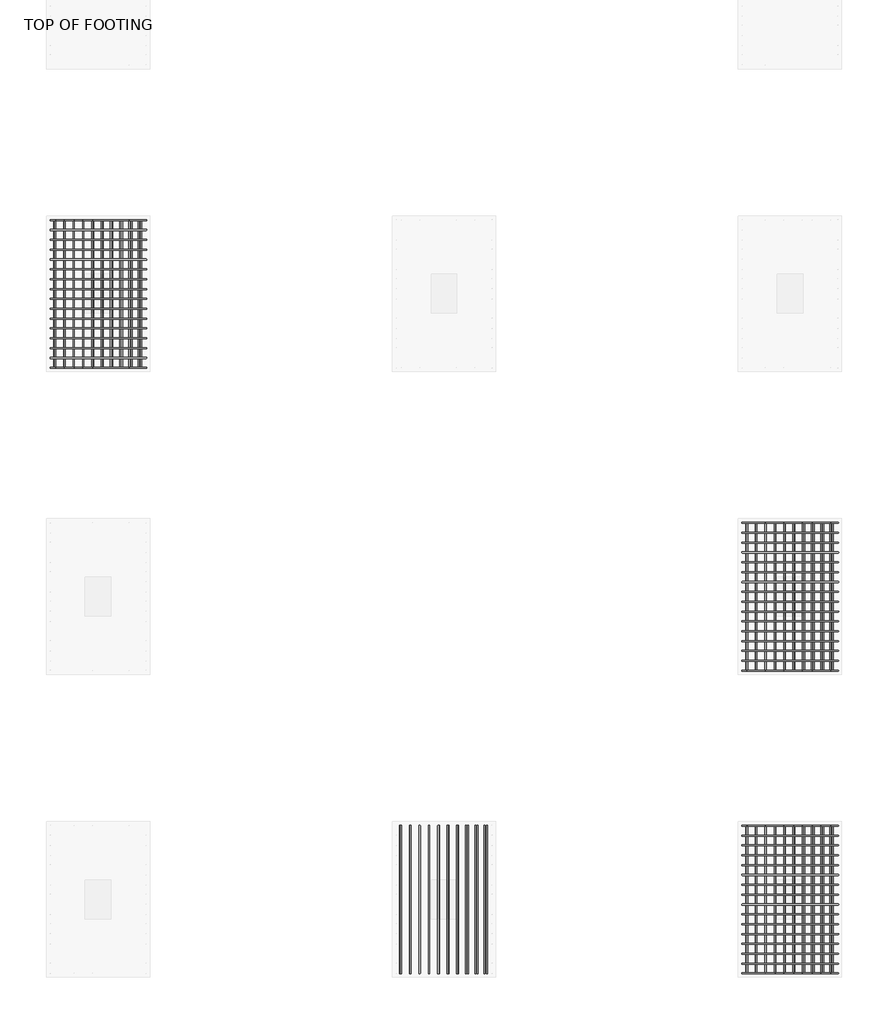
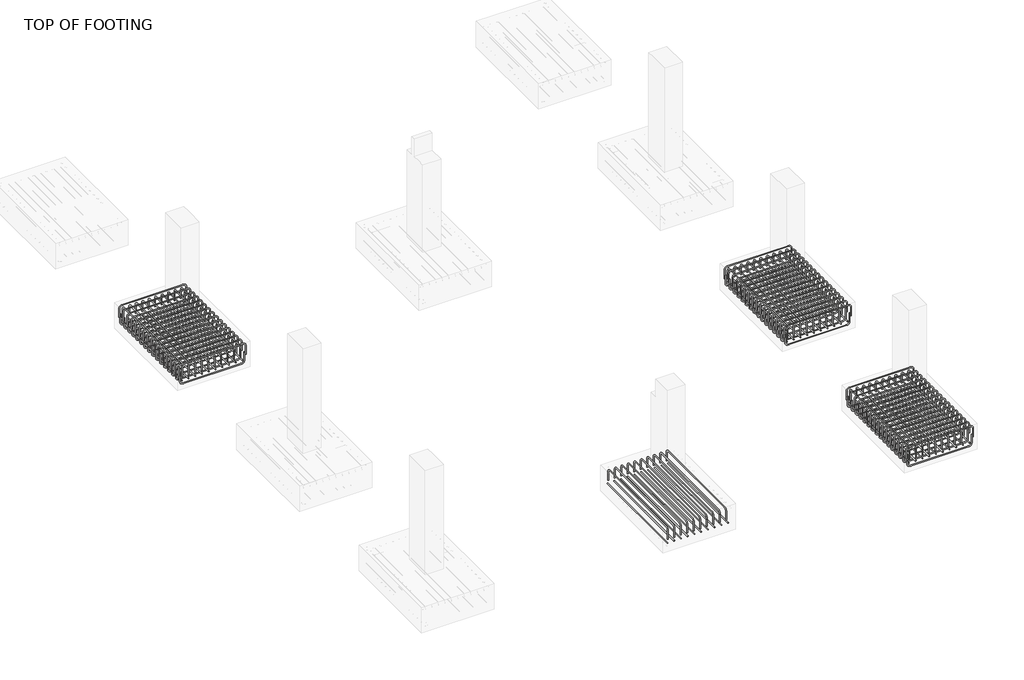
# One storey, part 6 of 8: 14 reinforcing bars.
"""IFC4 building model written with IfcOpenShell, lengths in millimetres."""

from ifc_helpers import new_model, si_unit, point, frame, origin, place, context, project, spatial, polyline, circle_curve, trimmed, segment, composite_curve, source, transform, mapped, element, save
from ifc_brep_helpers import swept_disk

model = new_model("IFC4")

# Units and contexts
model_context = context("Model", 3, world=origin())
ifc_project = project(units=[si_unit("LENGTHUNIT", "METRE", prefix="MILLI")], contexts=[model_context])

# Site, building, storey
site = spatial("IfcSite", under=ifc_project)
building = spatial("IfcBuilding", under=site)
storey = spatial("IfcBuildingStorey", under=building, Name="TOP OF FOOTING", Elevation=-1828.8)

# Reinforcing bars
placement = place(None, origin())
reinforcing_bar_shape = source(origin(), model_context, "Body", "SolidModel", [
    swept_disk(composite_curve([segment(polyline([(4698.4779803, 9626.3508557, -2021.4413313), (4698.4779803, 9626.3508557, -2168.7413313)]), True, "CONTINUOUS"), segment(trimmed(circle_curve(frame((4652.1279803, 9626.3508557, -2168.7413313), z_axis=(0.0, 1.0, 0.0), x_axis=(46.350000000000364, 0.0, 0.0)), 46.35), [point((4698.4779803, 9626.3508557, -2168.7413313))], [point((4652.1279803, 9626.3508557, -2215.0913313))], True, "CARTESIAN"), True, "CONTINUOUS"), segment(polyline([(4652.1279803, 9626.3508557, -2215.0913313), (3679.832969, 9626.3508557, -2215.0913313)]), True, "CONTINUOUS"), segment(trimmed(circle_curve(frame((3679.832969, 9626.3508557, -2168.7413313), z_axis=(0.0, 1.0, 0.0), x_axis=(0.0, 0.0, -46.34999999999991)), 46.35), [point((3679.832969, 9626.3508557, -2215.0913313))], [point((3633.482969, 9626.3508557, -2168.7413313))], True, "CARTESIAN"), True, "CONTINUOUS"), segment(polyline([(3633.482969, 9626.3508557, -2168.7413313), (3633.482969, 9626.3508557, -2021.4413313)]), True, "CONTINUOUS")], self_intersect=False), 6.35),
])
element("IfcReinforcingBar", 1, at=placement, inside=storey, context=model_context, shape_type="MappedRepresentation", body=[
    mapped(reinforcing_bar_shape, transform((0.0, 0.0, 0.0), x_axis=(1.0, 0.0, 0.0), y_axis=(0.0, 1.0, 0.0), z_axis=(0.0, 0.0, 1.0))),
    mapped(reinforcing_bar_shape, transform((0.0, -113.82, 0.0), x_axis=(1.0, 0.0, 0.0), y_axis=(0.0, 1.0, 0.0), z_axis=(0.0, 0.0, 1.0))),
    mapped(reinforcing_bar_shape, transform((0.0, -227.64, 0.0), x_axis=(1.0, 0.0, 0.0), y_axis=(0.0, 1.0, 0.0), z_axis=(0.0, 0.0, 1.0))),
    mapped(reinforcing_bar_shape, transform((0.0, -341.46, 0.0), x_axis=(1.0, 0.0, 0.0), y_axis=(0.0, 1.0, 0.0), z_axis=(0.0, 0.0, 1.0))),
    mapped(reinforcing_bar_shape, transform((0.0, -455.28, 0.0), x_axis=(1.0, 0.0, 0.0), y_axis=(0.0, 1.0, 0.0), z_axis=(0.0, 0.0, 1.0))),
    mapped(reinforcing_bar_shape, transform((0.0, -569.1, 0.0), x_axis=(1.0, 0.0, 0.0), y_axis=(0.0, 1.0, 0.0), z_axis=(0.0, 0.0, 1.0))),
    mapped(reinforcing_bar_shape, transform((0.0, -682.92, 0.0), x_axis=(1.0, 0.0, 0.0), y_axis=(0.0, 1.0, 0.0), z_axis=(0.0, 0.0, 1.0))),
    mapped(reinforcing_bar_shape, transform((0.0, -796.74, 0.0), x_axis=(1.0, 0.0, 0.0), y_axis=(0.0, 1.0, 0.0), z_axis=(0.0, 0.0, 1.0))),
    mapped(reinforcing_bar_shape, transform((0.0, -910.56, 0.0), x_axis=(1.0, 0.0, 0.0), y_axis=(0.0, 1.0, 0.0), z_axis=(0.0, 0.0, 1.0))),
    mapped(reinforcing_bar_shape, transform((0.0, -1024.38, 0.0), x_axis=(1.0, 0.0, 0.0), y_axis=(0.0, 1.0, 0.0), z_axis=(0.0, 0.0, 1.0))),
    mapped(reinforcing_bar_shape, transform((0.0, -1138.2, 0.0), x_axis=(1.0, 0.0, 0.0), y_axis=(0.0, 1.0, 0.0), z_axis=(0.0, 0.0, 1.0))),
    mapped(reinforcing_bar_shape, transform((0.0, -1252.02, 0.0), x_axis=(1.0, 0.0, 0.0), y_axis=(0.0, 1.0, 0.0), z_axis=(0.0, 0.0, 1.0))),
    mapped(reinforcing_bar_shape, transform((0.0, -1365.84, 0.0), x_axis=(1.0, 0.0, 0.0), y_axis=(0.0, 1.0, 0.0), z_axis=(0.0, 0.0, 1.0))),
    mapped(reinforcing_bar_shape, transform((0.0, -1479.66, 0.0), x_axis=(1.0, 0.0, 0.0), y_axis=(0.0, 1.0, 0.0), z_axis=(0.0, 0.0, 1.0))),
    mapped(reinforcing_bar_shape, transform((0.0, -1593.48, 0.0), x_axis=(1.0, 0.0, 0.0), y_axis=(0.0, 1.0, 0.0), z_axis=(0.0, 0.0, 1.0))),
    mapped(reinforcing_bar_shape, transform((0.0, -1707.3, 0.0), x_axis=(1.0, 0.0, 0.0), y_axis=(0.0, 1.0, 0.0), z_axis=(0.0, 0.0, 1.0))),
])
reinforcing_bar_2_shape = source(origin(), model_context, "Body", "SolidModel", [
    swept_disk(composite_curve([segment(polyline([(3615.6625983, 9626.3508557, -2068.8), (3615.6625983, 9626.3508557, -1921.5)]), True, "CONTINUOUS"), segment(trimmed(circle_curve(frame((3662.0125983, 9626.3508557, -1921.5), z_axis=(0.0, 1.0, 0.0), x_axis=(-46.34999999999991, 0.0, 0.0)), 46.35), [point((3615.6625983, 9626.3508557, -1921.5))], [point((3662.0125983, 9626.3508557, -1875.15))], True, "CARTESIAN"), True, "CONTINUOUS"), segment(polyline([(3662.0125983, 9626.3508557, -1875.15), (4676.6125983, 9626.3508557, -1875.15)]), True, "CONTINUOUS"), segment(trimmed(circle_curve(frame((4676.6125983, 9626.3508557, -1921.5), z_axis=(0.0, 1.0, 0.0), x_axis=(0.0, 0.0, 46.34999999999991)), 46.35), [point((4676.6125983, 9626.3508557, -1875.15))], [point((4722.9625983, 9626.3508557, -1921.5))], True, "CARTESIAN"), True, "CONTINUOUS"), segment(polyline([(4722.9625983, 9626.3508557, -1921.5), (4722.9625983, 9626.3508557, -2068.8)]), True, "CONTINUOUS")], self_intersect=False), 6.35),
])
element("IfcReinforcingBar", 2, at=placement, inside=storey, context=model_context, shape_type="MappedRepresentation", body=[
    mapped(reinforcing_bar_2_shape, transform((0.0, 0.0, 0.0), x_axis=(1.0, 0.0, 0.0), y_axis=(0.0, 1.0, 0.0), z_axis=(0.0, 0.0, 1.0))),
    mapped(reinforcing_bar_2_shape, transform((0.0, -113.82, 0.0), x_axis=(1.0, 0.0, 0.0), y_axis=(0.0, 1.0, 0.0), z_axis=(0.0, 0.0, 1.0))),
    mapped(reinforcing_bar_2_shape, transform((0.0, -227.64, 0.0), x_axis=(1.0, 0.0, 0.0), y_axis=(0.0, 1.0, 0.0), z_axis=(0.0, 0.0, 1.0))),
    mapped(reinforcing_bar_2_shape, transform((0.0, -341.46, 0.0), x_axis=(1.0, 0.0, 0.0), y_axis=(0.0, 1.0, 0.0), z_axis=(0.0, 0.0, 1.0))),
    mapped(reinforcing_bar_2_shape, transform((0.0, -455.28, 0.0), x_axis=(1.0, 0.0, 0.0), y_axis=(0.0, 1.0, 0.0), z_axis=(0.0, 0.0, 1.0))),
    mapped(reinforcing_bar_2_shape, transform((0.0, -569.1, 0.0), x_axis=(1.0, 0.0, 0.0), y_axis=(0.0, 1.0, 0.0), z_axis=(0.0, 0.0, 1.0))),
    mapped(reinforcing_bar_2_shape, transform((0.0, -682.92, 0.0), x_axis=(1.0, 0.0, 0.0), y_axis=(0.0, 1.0, 0.0), z_axis=(0.0, 0.0, 1.0))),
    mapped(reinforcing_bar_2_shape, transform((0.0, -796.74, 0.0), x_axis=(1.0, 0.0, 0.0), y_axis=(0.0, 1.0, 0.0), z_axis=(0.0, 0.0, 1.0))),
    mapped(reinforcing_bar_2_shape, transform((0.0, -910.56, 0.0), x_axis=(1.0, 0.0, 0.0), y_axis=(0.0, 1.0, 0.0), z_axis=(0.0, 0.0, 1.0))),
    mapped(reinforcing_bar_2_shape, transform((0.0, -1024.38, 0.0), x_axis=(1.0, 0.0, 0.0), y_axis=(0.0, 1.0, 0.0), z_axis=(0.0, 0.0, 1.0))),
    mapped(reinforcing_bar_2_shape, transform((0.0, -1138.2, 0.0), x_axis=(1.0, 0.0, 0.0), y_axis=(0.0, 1.0, 0.0), z_axis=(0.0, 0.0, 1.0))),
    mapped(reinforcing_bar_2_shape, transform((0.0, -1252.02, 0.0), x_axis=(1.0, 0.0, 0.0), y_axis=(0.0, 1.0, 0.0), z_axis=(0.0, 0.0, 1.0))),
    mapped(reinforcing_bar_2_shape, transform((0.0, -1365.84, 0.0), x_axis=(1.0, 0.0, 0.0), y_axis=(0.0, 1.0, 0.0), z_axis=(0.0, 0.0, 1.0))),
    mapped(reinforcing_bar_2_shape, transform((0.0, -1479.66, 0.0), x_axis=(1.0, 0.0, 0.0), y_axis=(0.0, 1.0, 0.0), z_axis=(0.0, 0.0, 1.0))),
    mapped(reinforcing_bar_2_shape, transform((0.0, -1593.48, 0.0), x_axis=(1.0, 0.0, 0.0), y_axis=(0.0, 1.0, 0.0), z_axis=(0.0, 0.0, 1.0))),
    mapped(reinforcing_bar_2_shape, transform((0.0, -1707.3, 0.0), x_axis=(1.0, 0.0, 0.0), y_axis=(0.0, 1.0, 0.0), z_axis=(0.0, 0.0, 1.0))),
])
reinforcing_bar_3_shape = source(origin(), model_context, "Body", "SolidModel", [
    swept_disk(composite_curve([segment(polyline([(3660.407291, 9632.7008557, -2155.1176129), (3660.407291, 7912.7008557, -2155.1176129)]), True, "CONTINUOUS")], self_intersect=False), 6.35),
])
element("IfcReinforcingBar", 3, at=placement, inside=storey, context=model_context, shape_type="MappedRepresentation", body=[
    mapped(reinforcing_bar_3_shape, transform((0.0, 0.0, 0.0), x_axis=(1.0, 0.0, 0.0), y_axis=(0.0, 1.0, 0.0), z_axis=(0.0, 0.0, 1.0))),
    mapped(reinforcing_bar_3_shape, transform((111.602188, 0.0, 0.0), x_axis=(1.0, 0.0, 0.0), y_axis=(0.0, 1.0, 0.0), z_axis=(0.0, 0.0, 1.0))),
    mapped(reinforcing_bar_3_shape, transform((223.2043759, 0.0, 0.0), x_axis=(1.0, 0.0, 0.0), y_axis=(0.0, 1.0, 0.0), z_axis=(0.0, 0.0, 1.0))),
    mapped(reinforcing_bar_3_shape, transform((334.8065639, 0.0, 0.0), x_axis=(1.0, 0.0, 0.0), y_axis=(0.0, 1.0, 0.0), z_axis=(0.0, 0.0, 1.0))),
    mapped(reinforcing_bar_3_shape, transform((446.4087519, 0.0, 0.0), x_axis=(1.0, 0.0, 0.0), y_axis=(0.0, 1.0, 0.0), z_axis=(0.0, 0.0, 1.0))),
    mapped(reinforcing_bar_3_shape, transform((558.0109398, 0.0, 0.0), x_axis=(1.0, 0.0, 0.0), y_axis=(0.0, 1.0, 0.0), z_axis=(0.0, 0.0, 1.0))),
    mapped(reinforcing_bar_3_shape, transform((669.6131278, 0.0, 0.0), x_axis=(1.0, 0.0, 0.0), y_axis=(0.0, 1.0, 0.0), z_axis=(0.0, 0.0, 1.0))),
    mapped(reinforcing_bar_3_shape, transform((781.2153158, 0.0, 0.0), x_axis=(1.0, 0.0, 0.0), y_axis=(0.0, 1.0, 0.0), z_axis=(0.0, 0.0, 1.0))),
    mapped(reinforcing_bar_3_shape, transform((892.8175037, 0.0, 0.0), x_axis=(1.0, 0.0, 0.0), y_axis=(0.0, 1.0, 0.0), z_axis=(0.0, 0.0, 1.0))),
    mapped(reinforcing_bar_3_shape, transform((1004.4196917, 0.0, 0.0), x_axis=(1.0, 0.0, 0.0), y_axis=(0.0, 1.0, 0.0), z_axis=(0.0, 0.0, 1.0))),
])
reinforcing_bar_4_shape = source(origin(), model_context, "Body", "SolidModel", [
    swept_disk(composite_curve([segment(polyline([(4635.7348019, 9626.3508557, -2094.6521303), (4635.7348019, 9626.3508557, -1947.3521303)]), True, "CONTINUOUS"), segment(trimmed(circle_curve(frame((4635.7348019, 9580.0008557, -1947.3521303), z_axis=(1.0, 0.0, 0.0), x_axis=(0.0, 46.350000000000364, 0.0)), 46.35), [point((4635.7348019, 9626.3508557, -1947.3521303))], [point((4635.7348019, 9580.0008557, -1901.0021303))], True, "CARTESIAN"), True, "CONTINUOUS"), segment(polyline([(4635.7348019, 9580.0008557, -1901.0021303), (4635.7348019, 7965.4008557, -1901.0021303)]), True, "CONTINUOUS"), segment(trimmed(circle_curve(frame((4635.7348019, 7965.4008557, -1947.3521303), z_axis=(1.0, 0.0, 0.0), x_axis=(0.0, 0.0, 46.34999999999991)), 46.35), [point((4635.7348019, 7965.4008557, -1901.0021303))], [point((4635.7348019, 7919.0508557, -1947.3521303))], True, "CARTESIAN"), True, "CONTINUOUS"), segment(polyline([(4635.7348019, 7919.0508557, -1947.3521303), (4635.7348019, 7919.0508557, -2094.6521303)]), True, "CONTINUOUS")], self_intersect=False), 6.35),
])
element("IfcReinforcingBar", 4, at=placement, inside=storey, context=model_context, shape_type="MappedRepresentation", body=[
    mapped(reinforcing_bar_4_shape, transform((0.0, 0.0, 0.0), x_axis=(1.0, 0.0, 0.0), y_axis=(0.0, 1.0, 0.0), z_axis=(0.0, 0.0, 1.0))),
    mapped(reinforcing_bar_4_shape, transform((-107.1680233, 0.0, 0.0), x_axis=(1.0, 0.0, 0.0), y_axis=(0.0, 1.0, 0.0), z_axis=(0.0, 0.0, 1.0))),
    mapped(reinforcing_bar_4_shape, transform((-214.3360466, 0.0, 0.0), x_axis=(1.0, 0.0, 0.0), y_axis=(0.0, 1.0, 0.0), z_axis=(0.0, 0.0, 1.0))),
    mapped(reinforcing_bar_4_shape, transform((-321.5040699, 0.0, 0.0), x_axis=(1.0, 0.0, 0.0), y_axis=(0.0, 1.0, 0.0), z_axis=(0.0, 0.0, 1.0))),
    mapped(reinforcing_bar_4_shape, transform((-428.6720932, 0.0, 0.0), x_axis=(1.0, 0.0, 0.0), y_axis=(0.0, 1.0, 0.0), z_axis=(0.0, 0.0, 1.0))),
    mapped(reinforcing_bar_4_shape, transform((-535.8401165, 0.0, 0.0), x_axis=(1.0, 0.0, 0.0), y_axis=(0.0, 1.0, 0.0), z_axis=(0.0, 0.0, 1.0))),
    mapped(reinforcing_bar_4_shape, transform((-643.0081398, 0.0, 0.0), x_axis=(1.0, 0.0, 0.0), y_axis=(0.0, 1.0, 0.0), z_axis=(0.0, 0.0, 1.0))),
    mapped(reinforcing_bar_4_shape, transform((-750.176163, 0.0, 0.0), x_axis=(1.0, 0.0, 0.0), y_axis=(0.0, 1.0, 0.0), z_axis=(0.0, 0.0, 1.0))),
    mapped(reinforcing_bar_4_shape, transform((-857.3441863, 0.0, 0.0), x_axis=(1.0, 0.0, 0.0), y_axis=(0.0, 1.0, 0.0), z_axis=(0.0, 0.0, 1.0))),
    mapped(reinforcing_bar_4_shape, transform((-964.5122096, 0.0, 0.0), x_axis=(1.0, 0.0, 0.0), y_axis=(0.0, 1.0, 0.0), z_axis=(0.0, 0.0, 1.0))),
])
reinforcing_bar_5_shape = source(origin(), model_context, "Body", "SolidModel", [
    swept_disk(composite_curve([segment(polyline([(7660.407291, 2632.7008557, -2155.1176129), (7660.407291, 912.7008557, -2155.1176129)]), True, "CONTINUOUS")], self_intersect=False), 6.35),
])
element("IfcReinforcingBar", 5, at=placement, inside=storey, context=model_context, shape_type="MappedRepresentation", body=[
    mapped(reinforcing_bar_5_shape, transform((0.0, 0.0, 0.0), x_axis=(1.0, 0.0, 0.0), y_axis=(0.0, 1.0, 0.0), z_axis=(0.0, 0.0, 1.0))),
    mapped(reinforcing_bar_5_shape, transform((111.602188, 0.0, 0.0), x_axis=(1.0, 0.0, 0.0), y_axis=(0.0, 1.0, 0.0), z_axis=(0.0, 0.0, 1.0))),
    mapped(reinforcing_bar_5_shape, transform((223.2043759, 0.0, 0.0), x_axis=(1.0, 0.0, 0.0), y_axis=(0.0, 1.0, 0.0), z_axis=(0.0, 0.0, 1.0))),
    mapped(reinforcing_bar_5_shape, transform((334.8065639, 0.0, 0.0), x_axis=(1.0, 0.0, 0.0), y_axis=(0.0, 1.0, 0.0), z_axis=(0.0, 0.0, 1.0))),
    mapped(reinforcing_bar_5_shape, transform((446.4087519, 0.0, 0.0), x_axis=(1.0, 0.0, 0.0), y_axis=(0.0, 1.0, 0.0), z_axis=(0.0, 0.0, 1.0))),
    mapped(reinforcing_bar_5_shape, transform((558.0109398, 0.0, 0.0), x_axis=(1.0, 0.0, 0.0), y_axis=(0.0, 1.0, 0.0), z_axis=(0.0, 0.0, 1.0))),
    mapped(reinforcing_bar_5_shape, transform((669.6131278, 0.0, 0.0), x_axis=(1.0, 0.0, 0.0), y_axis=(0.0, 1.0, 0.0), z_axis=(0.0, 0.0, 1.0))),
    mapped(reinforcing_bar_5_shape, transform((781.2153158, 0.0, 0.0), x_axis=(1.0, 0.0, 0.0), y_axis=(0.0, 1.0, 0.0), z_axis=(0.0, 0.0, 1.0))),
    mapped(reinforcing_bar_5_shape, transform((892.8175037, 0.0, 0.0), x_axis=(1.0, 0.0, 0.0), y_axis=(0.0, 1.0, 0.0), z_axis=(0.0, 0.0, 1.0))),
    mapped(reinforcing_bar_5_shape, transform((1004.4196917, 0.0, 0.0), x_axis=(1.0, 0.0, 0.0), y_axis=(0.0, 1.0, 0.0), z_axis=(0.0, 0.0, 1.0))),
])
reinforcing_bar_6_shape = source(origin(), model_context, "Body", "SolidModel", [
    swept_disk(composite_curve([segment(polyline([(8635.7348019, 2626.3508557, -2094.6521303), (8635.7348019, 2626.3508557, -1947.3521303)]), True, "CONTINUOUS"), segment(trimmed(circle_curve(frame((8635.7348019, 2580.0008557, -1947.3521303), z_axis=(1.0, 0.0, 0.0), x_axis=(0.0, 46.34999999999991, 0.0)), 46.35), [point((8635.7348019, 2626.3508557, -1947.3521303))], [point((8635.7348019, 2580.0008557, -1901.0021303))], True, "CARTESIAN"), True, "CONTINUOUS"), segment(polyline([(8635.7348019, 2580.0008557, -1901.0021303), (8635.7348019, 965.4008557, -1901.0021303)]), True, "CONTINUOUS"), segment(trimmed(circle_curve(frame((8635.7348019, 965.4008557, -1947.3521303), z_axis=(1.0, 0.0, 0.0), x_axis=(0.0, 0.0, 46.34999999999991)), 46.35), [point((8635.7348019, 965.4008557, -1901.0021303))], [point((8635.7348019, 919.0508557, -1947.3521303))], True, "CARTESIAN"), True, "CONTINUOUS"), segment(polyline([(8635.7348019, 919.0508557, -1947.3521303), (8635.7348019, 919.0508557, -2094.6521303)]), True, "CONTINUOUS")], self_intersect=False), 6.35),
])
element("IfcReinforcingBar", 6, at=placement, inside=storey, context=model_context, shape_type="MappedRepresentation", body=[
    mapped(reinforcing_bar_6_shape, transform((0.0, 0.0, 0.0), x_axis=(1.0, 0.0, 0.0), y_axis=(0.0, 1.0, 0.0), z_axis=(0.0, 0.0, 1.0))),
    mapped(reinforcing_bar_6_shape, transform((-107.1680233, 0.0, 0.0), x_axis=(1.0, 0.0, 0.0), y_axis=(0.0, 1.0, 0.0), z_axis=(0.0, 0.0, 1.0))),
    mapped(reinforcing_bar_6_shape, transform((-214.3360466, 0.0, 0.0), x_axis=(1.0, 0.0, 0.0), y_axis=(0.0, 1.0, 0.0), z_axis=(0.0, 0.0, 1.0))),
    mapped(reinforcing_bar_6_shape, transform((-321.5040699, 0.0, 0.0), x_axis=(1.0, 0.0, 0.0), y_axis=(0.0, 1.0, 0.0), z_axis=(0.0, 0.0, 1.0))),
    mapped(reinforcing_bar_6_shape, transform((-428.6720932, 0.0, 0.0), x_axis=(1.0, 0.0, 0.0), y_axis=(0.0, 1.0, 0.0), z_axis=(0.0, 0.0, 1.0))),
    mapped(reinforcing_bar_6_shape, transform((-535.8401165, 0.0, 0.0), x_axis=(1.0, 0.0, 0.0), y_axis=(0.0, 1.0, 0.0), z_axis=(0.0, 0.0, 1.0))),
    mapped(reinforcing_bar_6_shape, transform((-643.0081398, 0.0, 0.0), x_axis=(1.0, 0.0, 0.0), y_axis=(0.0, 1.0, 0.0), z_axis=(0.0, 0.0, 1.0))),
    mapped(reinforcing_bar_6_shape, transform((-750.176163, 0.0, 0.0), x_axis=(1.0, 0.0, 0.0), y_axis=(0.0, 1.0, 0.0), z_axis=(0.0, 0.0, 1.0))),
    mapped(reinforcing_bar_6_shape, transform((-857.3441863, 0.0, 0.0), x_axis=(1.0, 0.0, 0.0), y_axis=(0.0, 1.0, 0.0), z_axis=(0.0, 0.0, 1.0))),
    mapped(reinforcing_bar_6_shape, transform((-964.5122096, 0.0, 0.0), x_axis=(1.0, 0.0, 0.0), y_axis=(0.0, 1.0, 0.0), z_axis=(0.0, 0.0, 1.0))),
])
reinforcing_bar_7_shape = source(origin(), model_context, "Body", "SolidModel", [
    swept_disk(composite_curve([segment(polyline([(12698.4779803, 6126.3508557, -2021.4413313), (12698.4779803, 6126.3508557, -2168.7413313)]), True, "CONTINUOUS"), segment(trimmed(circle_curve(frame((12652.1279803, 6126.3508557, -2168.7413313), z_axis=(0.0, 1.0, 0.0), x_axis=(46.350000000000364, 0.0, 0.0)), 46.35), [point((12698.4779803, 6126.3508557, -2168.7413313))], [point((12652.1279803, 6126.3508557, -2215.0913313))], True, "CARTESIAN"), True, "CONTINUOUS"), segment(polyline([(12652.1279803, 6126.3508557, -2215.0913313), (11679.832969, 6126.3508557, -2215.0913313)]), True, "CONTINUOUS"), segment(trimmed(circle_curve(frame((11679.832969, 6126.3508557, -2168.7413313), z_axis=(0.0, 1.0, 0.0), x_axis=(0.0, 0.0, -46.34999999999991)), 46.35), [point((11679.832969, 6126.3508557, -2215.0913313))], [point((11633.482969, 6126.3508557, -2168.7413313))], True, "CARTESIAN"), True, "CONTINUOUS"), segment(polyline([(11633.482969, 6126.3508557, -2168.7413313), (11633.482969, 6126.3508557, -2021.4413313)]), True, "CONTINUOUS")], self_intersect=False), 6.35),
])
element("IfcReinforcingBar", 7, at=placement, inside=storey, context=model_context, shape_type="MappedRepresentation", body=[
    mapped(reinforcing_bar_7_shape, transform((0.0, 0.0, 0.0), x_axis=(1.0, 0.0, 0.0), y_axis=(0.0, 1.0, 0.0), z_axis=(0.0, 0.0, 1.0))),
    mapped(reinforcing_bar_7_shape, transform((0.0, -113.82, 0.0), x_axis=(1.0, 0.0, 0.0), y_axis=(0.0, 1.0, 0.0), z_axis=(0.0, 0.0, 1.0))),
    mapped(reinforcing_bar_7_shape, transform((0.0, -227.64, 0.0), x_axis=(1.0, 0.0, 0.0), y_axis=(0.0, 1.0, 0.0), z_axis=(0.0, 0.0, 1.0))),
    mapped(reinforcing_bar_7_shape, transform((0.0, -341.46, 0.0), x_axis=(1.0, 0.0, 0.0), y_axis=(0.0, 1.0, 0.0), z_axis=(0.0, 0.0, 1.0))),
    mapped(reinforcing_bar_7_shape, transform((0.0, -455.28, 0.0), x_axis=(1.0, 0.0, 0.0), y_axis=(0.0, 1.0, 0.0), z_axis=(0.0, 0.0, 1.0))),
    mapped(reinforcing_bar_7_shape, transform((0.0, -569.1, 0.0), x_axis=(1.0, 0.0, 0.0), y_axis=(0.0, 1.0, 0.0), z_axis=(0.0, 0.0, 1.0))),
    mapped(reinforcing_bar_7_shape, transform((0.0, -682.92, 0.0), x_axis=(1.0, 0.0, 0.0), y_axis=(0.0, 1.0, 0.0), z_axis=(0.0, 0.0, 1.0))),
    mapped(reinforcing_bar_7_shape, transform((0.0, -796.74, 0.0), x_axis=(1.0, 0.0, 0.0), y_axis=(0.0, 1.0, 0.0), z_axis=(0.0, 0.0, 1.0))),
    mapped(reinforcing_bar_7_shape, transform((0.0, -910.56, 0.0), x_axis=(1.0, 0.0, 0.0), y_axis=(0.0, 1.0, 0.0), z_axis=(0.0, 0.0, 1.0))),
    mapped(reinforcing_bar_7_shape, transform((0.0, -1024.38, 0.0), x_axis=(1.0, 0.0, 0.0), y_axis=(0.0, 1.0, 0.0), z_axis=(0.0, 0.0, 1.0))),
    mapped(reinforcing_bar_7_shape, transform((0.0, -1138.2, 0.0), x_axis=(1.0, 0.0, 0.0), y_axis=(0.0, 1.0, 0.0), z_axis=(0.0, 0.0, 1.0))),
    mapped(reinforcing_bar_7_shape, transform((0.0, -1252.02, 0.0), x_axis=(1.0, 0.0, 0.0), y_axis=(0.0, 1.0, 0.0), z_axis=(0.0, 0.0, 1.0))),
    mapped(reinforcing_bar_7_shape, transform((0.0, -1365.84, 0.0), x_axis=(1.0, 0.0, 0.0), y_axis=(0.0, 1.0, 0.0), z_axis=(0.0, 0.0, 1.0))),
    mapped(reinforcing_bar_7_shape, transform((0.0, -1479.66, 0.0), x_axis=(1.0, 0.0, 0.0), y_axis=(0.0, 1.0, 0.0), z_axis=(0.0, 0.0, 1.0))),
    mapped(reinforcing_bar_7_shape, transform((0.0, -1593.48, 0.0), x_axis=(1.0, 0.0, 0.0), y_axis=(0.0, 1.0, 0.0), z_axis=(0.0, 0.0, 1.0))),
    mapped(reinforcing_bar_7_shape, transform((0.0, -1707.3, 0.0), x_axis=(1.0, 0.0, 0.0), y_axis=(0.0, 1.0, 0.0), z_axis=(0.0, 0.0, 1.0))),
])
reinforcing_bar_8_shape = source(origin(), model_context, "Body", "SolidModel", [
    swept_disk(composite_curve([segment(polyline([(11615.6625983, 6126.3508557, -2068.8), (11615.6625983, 6126.3508557, -1921.5)]), True, "CONTINUOUS"), segment(trimmed(circle_curve(frame((11662.0125983, 6126.3508557, -1921.5), z_axis=(0.0, 1.0, 0.0), x_axis=(-46.350000000000364, 0.0, 0.0)), 46.35), [point((11615.6625983, 6126.3508557, -1921.5))], [point((11662.0125983, 6126.3508557, -1875.15))], True, "CARTESIAN"), True, "CONTINUOUS"), segment(polyline([(11662.0125983, 6126.3508557, -1875.15), (12676.6125983, 6126.3508557, -1875.15)]), True, "CONTINUOUS"), segment(trimmed(circle_curve(frame((12676.6125983, 6126.3508557, -1921.5), z_axis=(0.0, 1.0, 0.0), x_axis=(0.0, 0.0, 46.34999999999991)), 46.35), [point((12676.6125983, 6126.3508557, -1875.15))], [point((12722.9625983, 6126.3508557, -1921.5))], True, "CARTESIAN"), True, "CONTINUOUS"), segment(polyline([(12722.9625983, 6126.3508557, -1921.5), (12722.9625983, 6126.3508557, -2068.8)]), True, "CONTINUOUS")], self_intersect=False), 6.35),
])
element("IfcReinforcingBar", 8, at=placement, inside=storey, context=model_context, shape_type="MappedRepresentation", body=[
    mapped(reinforcing_bar_8_shape, transform((0.0, 0.0, 0.0), x_axis=(1.0, 0.0, 0.0), y_axis=(0.0, 1.0, 0.0), z_axis=(0.0, 0.0, 1.0))),
    mapped(reinforcing_bar_8_shape, transform((0.0, -113.82, 0.0), x_axis=(1.0, 0.0, 0.0), y_axis=(0.0, 1.0, 0.0), z_axis=(0.0, 0.0, 1.0))),
    mapped(reinforcing_bar_8_shape, transform((0.0, -227.64, 0.0), x_axis=(1.0, 0.0, 0.0), y_axis=(0.0, 1.0, 0.0), z_axis=(0.0, 0.0, 1.0))),
    mapped(reinforcing_bar_8_shape, transform((0.0, -341.46, 0.0), x_axis=(1.0, 0.0, 0.0), y_axis=(0.0, 1.0, 0.0), z_axis=(0.0, 0.0, 1.0))),
    mapped(reinforcing_bar_8_shape, transform((0.0, -455.28, 0.0), x_axis=(1.0, 0.0, 0.0), y_axis=(0.0, 1.0, 0.0), z_axis=(0.0, 0.0, 1.0))),
    mapped(reinforcing_bar_8_shape, transform((0.0, -569.1, 0.0), x_axis=(1.0, 0.0, 0.0), y_axis=(0.0, 1.0, 0.0), z_axis=(0.0, 0.0, 1.0))),
    mapped(reinforcing_bar_8_shape, transform((0.0, -682.92, 0.0), x_axis=(1.0, 0.0, 0.0), y_axis=(0.0, 1.0, 0.0), z_axis=(0.0, 0.0, 1.0))),
    mapped(reinforcing_bar_8_shape, transform((0.0, -796.74, 0.0), x_axis=(1.0, 0.0, 0.0), y_axis=(0.0, 1.0, 0.0), z_axis=(0.0, 0.0, 1.0))),
    mapped(reinforcing_bar_8_shape, transform((0.0, -910.56, 0.0), x_axis=(1.0, 0.0, 0.0), y_axis=(0.0, 1.0, 0.0), z_axis=(0.0, 0.0, 1.0))),
    mapped(reinforcing_bar_8_shape, transform((0.0, -1024.38, 0.0), x_axis=(1.0, 0.0, 0.0), y_axis=(0.0, 1.0, 0.0), z_axis=(0.0, 0.0, 1.0))),
    mapped(reinforcing_bar_8_shape, transform((0.0, -1138.2, 0.0), x_axis=(1.0, 0.0, 0.0), y_axis=(0.0, 1.0, 0.0), z_axis=(0.0, 0.0, 1.0))),
    mapped(reinforcing_bar_8_shape, transform((0.0, -1252.02, 0.0), x_axis=(1.0, 0.0, 0.0), y_axis=(0.0, 1.0, 0.0), z_axis=(0.0, 0.0, 1.0))),
    mapped(reinforcing_bar_8_shape, transform((0.0, -1365.84, 0.0), x_axis=(1.0, 0.0, 0.0), y_axis=(0.0, 1.0, 0.0), z_axis=(0.0, 0.0, 1.0))),
    mapped(reinforcing_bar_8_shape, transform((0.0, -1479.66, 0.0), x_axis=(1.0, 0.0, 0.0), y_axis=(0.0, 1.0, 0.0), z_axis=(0.0, 0.0, 1.0))),
    mapped(reinforcing_bar_8_shape, transform((0.0, -1593.48, 0.0), x_axis=(1.0, 0.0, 0.0), y_axis=(0.0, 1.0, 0.0), z_axis=(0.0, 0.0, 1.0))),
    mapped(reinforcing_bar_8_shape, transform((0.0, -1707.3, 0.0), x_axis=(1.0, 0.0, 0.0), y_axis=(0.0, 1.0, 0.0), z_axis=(0.0, 0.0, 1.0))),
])
reinforcing_bar_9_shape = source(origin(), model_context, "Body", "SolidModel", [
    swept_disk(composite_curve([segment(polyline([(11660.407291, 6132.7008557, -2155.1176129), (11660.407291, 4412.7008557, -2155.1176129)]), True, "CONTINUOUS")], self_intersect=False), 6.35),
])
element("IfcReinforcingBar", 9, at=placement, inside=storey, context=model_context, shape_type="MappedRepresentation", body=[
    mapped(reinforcing_bar_9_shape, transform((0.0, 0.0, 0.0), x_axis=(1.0, 0.0, 0.0), y_axis=(0.0, 1.0, 0.0), z_axis=(0.0, 0.0, 1.0))),
    mapped(reinforcing_bar_9_shape, transform((111.602188, 0.0, 0.0), x_axis=(1.0, 0.0, 0.0), y_axis=(0.0, 1.0, 0.0), z_axis=(0.0, 0.0, 1.0))),
    mapped(reinforcing_bar_9_shape, transform((223.2043759, 0.0, 0.0), x_axis=(1.0, 0.0, 0.0), y_axis=(0.0, 1.0, 0.0), z_axis=(0.0, 0.0, 1.0))),
    mapped(reinforcing_bar_9_shape, transform((334.8065639, 0.0, 0.0), x_axis=(1.0, 0.0, 0.0), y_axis=(0.0, 1.0, 0.0), z_axis=(0.0, 0.0, 1.0))),
    mapped(reinforcing_bar_9_shape, transform((446.4087519, 0.0, 0.0), x_axis=(1.0, 0.0, 0.0), y_axis=(0.0, 1.0, 0.0), z_axis=(0.0, 0.0, 1.0))),
    mapped(reinforcing_bar_9_shape, transform((558.0109398, 0.0, 0.0), x_axis=(1.0, 0.0, 0.0), y_axis=(0.0, 1.0, 0.0), z_axis=(0.0, 0.0, 1.0))),
    mapped(reinforcing_bar_9_shape, transform((669.6131278, 0.0, 0.0), x_axis=(1.0, 0.0, 0.0), y_axis=(0.0, 1.0, 0.0), z_axis=(0.0, 0.0, 1.0))),
    mapped(reinforcing_bar_9_shape, transform((781.2153158, 0.0, 0.0), x_axis=(1.0, 0.0, 0.0), y_axis=(0.0, 1.0, 0.0), z_axis=(0.0, 0.0, 1.0))),
    mapped(reinforcing_bar_9_shape, transform((892.8175037, 0.0, 0.0), x_axis=(1.0, 0.0, 0.0), y_axis=(0.0, 1.0, 0.0), z_axis=(0.0, 0.0, 1.0))),
    mapped(reinforcing_bar_9_shape, transform((1004.4196917, 0.0, 0.0), x_axis=(1.0, 0.0, 0.0), y_axis=(0.0, 1.0, 0.0), z_axis=(0.0, 0.0, 1.0))),
])
reinforcing_bar_10_shape = source(origin(), model_context, "Body", "SolidModel", [
    swept_disk(composite_curve([segment(polyline([(12635.7348019, 6126.3508557, -2094.6521303), (12635.7348019, 6126.3508557, -1947.3521303)]), True, "CONTINUOUS"), segment(trimmed(circle_curve(frame((12635.7348019, 6080.0008557, -1947.3521303), z_axis=(1.0, 0.0, 0.0), x_axis=(0.0, 46.349999999999454, 0.0)), 46.35), [point((12635.7348019, 6126.3508557, -1947.3521303))], [point((12635.7348019, 6080.0008557, -1901.0021303))], True, "CARTESIAN"), True, "CONTINUOUS"), segment(polyline([(12635.7348019, 6080.0008557, -1901.0021303), (12635.7348019, 4465.4008557, -1901.0021303)]), True, "CONTINUOUS"), segment(trimmed(circle_curve(frame((12635.7348019, 4465.4008557, -1947.3521303), z_axis=(1.0, 0.0, 0.0), x_axis=(0.0, 0.0, 46.34999999999991)), 46.35), [point((12635.7348019, 4465.4008557, -1901.0021303))], [point((12635.7348019, 4419.0508557, -1947.3521303))], True, "CARTESIAN"), True, "CONTINUOUS"), segment(polyline([(12635.7348019, 4419.0508557, -1947.3521303), (12635.7348019, 4419.0508557, -2094.6521303)]), True, "CONTINUOUS")], self_intersect=False), 6.35),
])
element("IfcReinforcingBar", 10, at=placement, inside=storey, context=model_context, shape_type="MappedRepresentation", body=[
    mapped(reinforcing_bar_10_shape, transform((0.0, 0.0, 0.0), x_axis=(1.0, 0.0, 0.0), y_axis=(0.0, 1.0, 0.0), z_axis=(0.0, 0.0, 1.0))),
    mapped(reinforcing_bar_10_shape, transform((-107.1680233, 0.0, 0.0), x_axis=(1.0, 0.0, 0.0), y_axis=(0.0, 1.0, 0.0), z_axis=(0.0, 0.0, 1.0))),
    mapped(reinforcing_bar_10_shape, transform((-214.3360466, 0.0, 0.0), x_axis=(1.0, 0.0, 0.0), y_axis=(0.0, 1.0, 0.0), z_axis=(0.0, 0.0, 1.0))),
    mapped(reinforcing_bar_10_shape, transform((-321.5040699, 0.0, 0.0), x_axis=(1.0, 0.0, 0.0), y_axis=(0.0, 1.0, 0.0), z_axis=(0.0, 0.0, 1.0))),
    mapped(reinforcing_bar_10_shape, transform((-428.6720932, 0.0, 0.0), x_axis=(1.0, 0.0, 0.0), y_axis=(0.0, 1.0, 0.0), z_axis=(0.0, 0.0, 1.0))),
    mapped(reinforcing_bar_10_shape, transform((-535.8401165, 0.0, 0.0), x_axis=(1.0, 0.0, 0.0), y_axis=(0.0, 1.0, 0.0), z_axis=(0.0, 0.0, 1.0))),
    mapped(reinforcing_bar_10_shape, transform((-643.0081398, 0.0, 0.0), x_axis=(1.0, 0.0, 0.0), y_axis=(0.0, 1.0, 0.0), z_axis=(0.0, 0.0, 1.0))),
    mapped(reinforcing_bar_10_shape, transform((-750.176163, 0.0, 0.0), x_axis=(1.0, 0.0, 0.0), y_axis=(0.0, 1.0, 0.0), z_axis=(0.0, 0.0, 1.0))),
    mapped(reinforcing_bar_10_shape, transform((-857.3441863, 0.0, 0.0), x_axis=(1.0, 0.0, 0.0), y_axis=(0.0, 1.0, 0.0), z_axis=(0.0, 0.0, 1.0))),
    mapped(reinforcing_bar_10_shape, transform((-964.5122096, 0.0, 0.0), x_axis=(1.0, 0.0, 0.0), y_axis=(0.0, 1.0, 0.0), z_axis=(0.0, 0.0, 1.0))),
])
reinforcing_bar_11_shape = source(origin(), model_context, "Body", "SolidModel", [
    swept_disk(composite_curve([segment(polyline([(12698.4779803, 2626.3508557, -2021.4413313), (12698.4779803, 2626.3508557, -2168.7413313)]), True, "CONTINUOUS"), segment(trimmed(circle_curve(frame((12652.1279803, 2626.3508557, -2168.7413313), z_axis=(0.0, 1.0, 0.0), x_axis=(46.350000000000364, 0.0, 0.0)), 46.35), [point((12698.4779803, 2626.3508557, -2168.7413313))], [point((12652.1279803, 2626.3508557, -2215.0913313))], True, "CARTESIAN"), True, "CONTINUOUS"), segment(polyline([(12652.1279803, 2626.3508557, -2215.0913313), (11679.832969, 2626.3508557, -2215.0913313)]), True, "CONTINUOUS"), segment(trimmed(circle_curve(frame((11679.832969, 2626.3508557, -2168.7413313), z_axis=(0.0, 1.0, 0.0), x_axis=(0.0, 0.0, -46.34999999999991)), 46.35), [point((11679.832969, 2626.3508557, -2215.0913313))], [point((11633.482969, 2626.3508557, -2168.7413313))], True, "CARTESIAN"), True, "CONTINUOUS"), segment(polyline([(11633.482969, 2626.3508557, -2168.7413313), (11633.482969, 2626.3508557, -2021.4413313)]), True, "CONTINUOUS")], self_intersect=False), 6.35),
])
element("IfcReinforcingBar", 11, at=placement, inside=storey, context=model_context, shape_type="MappedRepresentation", body=[
    mapped(reinforcing_bar_11_shape, transform((0.0, 0.0, 0.0), x_axis=(1.0, 0.0, 0.0), y_axis=(0.0, 1.0, 0.0), z_axis=(0.0, 0.0, 1.0))),
    mapped(reinforcing_bar_11_shape, transform((0.0, -113.82, 0.0), x_axis=(1.0, 0.0, 0.0), y_axis=(0.0, 1.0, 0.0), z_axis=(0.0, 0.0, 1.0))),
    mapped(reinforcing_bar_11_shape, transform((0.0, -227.64, 0.0), x_axis=(1.0, 0.0, 0.0), y_axis=(0.0, 1.0, 0.0), z_axis=(0.0, 0.0, 1.0))),
    mapped(reinforcing_bar_11_shape, transform((0.0, -341.46, 0.0), x_axis=(1.0, 0.0, 0.0), y_axis=(0.0, 1.0, 0.0), z_axis=(0.0, 0.0, 1.0))),
    mapped(reinforcing_bar_11_shape, transform((0.0, -455.28, 0.0), x_axis=(1.0, 0.0, 0.0), y_axis=(0.0, 1.0, 0.0), z_axis=(0.0, 0.0, 1.0))),
    mapped(reinforcing_bar_11_shape, transform((0.0, -569.1, 0.0), x_axis=(1.0, 0.0, 0.0), y_axis=(0.0, 1.0, 0.0), z_axis=(0.0, 0.0, 1.0))),
    mapped(reinforcing_bar_11_shape, transform((0.0, -682.92, 0.0), x_axis=(1.0, 0.0, 0.0), y_axis=(0.0, 1.0, 0.0), z_axis=(0.0, 0.0, 1.0))),
    mapped(reinforcing_bar_11_shape, transform((0.0, -796.74, 0.0), x_axis=(1.0, 0.0, 0.0), y_axis=(0.0, 1.0, 0.0), z_axis=(0.0, 0.0, 1.0))),
    mapped(reinforcing_bar_11_shape, transform((0.0, -910.56, 0.0), x_axis=(1.0, 0.0, 0.0), y_axis=(0.0, 1.0, 0.0), z_axis=(0.0, 0.0, 1.0))),
    mapped(reinforcing_bar_11_shape, transform((0.0, -1024.38, 0.0), x_axis=(1.0, 0.0, 0.0), y_axis=(0.0, 1.0, 0.0), z_axis=(0.0, 0.0, 1.0))),
    mapped(reinforcing_bar_11_shape, transform((0.0, -1138.2, 0.0), x_axis=(1.0, 0.0, 0.0), y_axis=(0.0, 1.0, 0.0), z_axis=(0.0, 0.0, 1.0))),
    mapped(reinforcing_bar_11_shape, transform((0.0, -1252.02, 0.0), x_axis=(1.0, 0.0, 0.0), y_axis=(0.0, 1.0, 0.0), z_axis=(0.0, 0.0, 1.0))),
    mapped(reinforcing_bar_11_shape, transform((0.0, -1365.84, 0.0), x_axis=(1.0, 0.0, 0.0), y_axis=(0.0, 1.0, 0.0), z_axis=(0.0, 0.0, 1.0))),
    mapped(reinforcing_bar_11_shape, transform((0.0, -1479.66, 0.0), x_axis=(1.0, 0.0, 0.0), y_axis=(0.0, 1.0, 0.0), z_axis=(0.0, 0.0, 1.0))),
    mapped(reinforcing_bar_11_shape, transform((0.0, -1593.48, 0.0), x_axis=(1.0, 0.0, 0.0), y_axis=(0.0, 1.0, 0.0), z_axis=(0.0, 0.0, 1.0))),
    mapped(reinforcing_bar_11_shape, transform((0.0, -1707.3, 0.0), x_axis=(1.0, 0.0, 0.0), y_axis=(0.0, 1.0, 0.0), z_axis=(0.0, 0.0, 1.0))),
])
reinforcing_bar_12_shape = source(origin(), model_context, "Body", "SolidModel", [
    swept_disk(composite_curve([segment(polyline([(11615.6625983, 2626.3508557, -2068.8), (11615.6625983, 2626.3508557, -1921.5)]), True, "CONTINUOUS"), segment(trimmed(circle_curve(frame((11662.0125983, 2626.3508557, -1921.5), z_axis=(0.0, 1.0, 0.0), x_axis=(-46.350000000000364, 0.0, 0.0)), 46.35), [point((11615.6625983, 2626.3508557, -1921.5))], [point((11662.0125983, 2626.3508557, -1875.15))], True, "CARTESIAN"), True, "CONTINUOUS"), segment(polyline([(11662.0125983, 2626.3508557, -1875.15), (12676.6125983, 2626.3508557, -1875.15)]), True, "CONTINUOUS"), segment(trimmed(circle_curve(frame((12676.6125983, 2626.3508557, -1921.5), z_axis=(0.0, 1.0, 0.0), x_axis=(0.0, 0.0, 46.34999999999991)), 46.35), [point((12676.6125983, 2626.3508557, -1875.15))], [point((12722.9625983, 2626.3508557, -1921.5))], True, "CARTESIAN"), True, "CONTINUOUS"), segment(polyline([(12722.9625983, 2626.3508557, -1921.5), (12722.9625983, 2626.3508557, -2068.8)]), True, "CONTINUOUS")], self_intersect=False), 6.35),
])
element("IfcReinforcingBar", 12, at=placement, inside=storey, context=model_context, shape_type="MappedRepresentation", body=[
    mapped(reinforcing_bar_12_shape, transform((0.0, 0.0, 0.0), x_axis=(1.0, 0.0, 0.0), y_axis=(0.0, 1.0, 0.0), z_axis=(0.0, 0.0, 1.0))),
    mapped(reinforcing_bar_12_shape, transform((0.0, -113.82, 0.0), x_axis=(1.0, 0.0, 0.0), y_axis=(0.0, 1.0, 0.0), z_axis=(0.0, 0.0, 1.0))),
    mapped(reinforcing_bar_12_shape, transform((0.0, -227.64, 0.0), x_axis=(1.0, 0.0, 0.0), y_axis=(0.0, 1.0, 0.0), z_axis=(0.0, 0.0, 1.0))),
    mapped(reinforcing_bar_12_shape, transform((0.0, -341.46, 0.0), x_axis=(1.0, 0.0, 0.0), y_axis=(0.0, 1.0, 0.0), z_axis=(0.0, 0.0, 1.0))),
    mapped(reinforcing_bar_12_shape, transform((0.0, -455.28, 0.0), x_axis=(1.0, 0.0, 0.0), y_axis=(0.0, 1.0, 0.0), z_axis=(0.0, 0.0, 1.0))),
    mapped(reinforcing_bar_12_shape, transform((0.0, -569.1, 0.0), x_axis=(1.0, 0.0, 0.0), y_axis=(0.0, 1.0, 0.0), z_axis=(0.0, 0.0, 1.0))),
    mapped(reinforcing_bar_12_shape, transform((0.0, -682.92, 0.0), x_axis=(1.0, 0.0, 0.0), y_axis=(0.0, 1.0, 0.0), z_axis=(0.0, 0.0, 1.0))),
    mapped(reinforcing_bar_12_shape, transform((0.0, -796.74, 0.0), x_axis=(1.0, 0.0, 0.0), y_axis=(0.0, 1.0, 0.0), z_axis=(0.0, 0.0, 1.0))),
    mapped(reinforcing_bar_12_shape, transform((0.0, -910.56, 0.0), x_axis=(1.0, 0.0, 0.0), y_axis=(0.0, 1.0, 0.0), z_axis=(0.0, 0.0, 1.0))),
    mapped(reinforcing_bar_12_shape, transform((0.0, -1024.38, 0.0), x_axis=(1.0, 0.0, 0.0), y_axis=(0.0, 1.0, 0.0), z_axis=(0.0, 0.0, 1.0))),
    mapped(reinforcing_bar_12_shape, transform((0.0, -1138.2, 0.0), x_axis=(1.0, 0.0, 0.0), y_axis=(0.0, 1.0, 0.0), z_axis=(0.0, 0.0, 1.0))),
    mapped(reinforcing_bar_12_shape, transform((0.0, -1252.02, 0.0), x_axis=(1.0, 0.0, 0.0), y_axis=(0.0, 1.0, 0.0), z_axis=(0.0, 0.0, 1.0))),
    mapped(reinforcing_bar_12_shape, transform((0.0, -1365.84, 0.0), x_axis=(1.0, 0.0, 0.0), y_axis=(0.0, 1.0, 0.0), z_axis=(0.0, 0.0, 1.0))),
    mapped(reinforcing_bar_12_shape, transform((0.0, -1479.66, 0.0), x_axis=(1.0, 0.0, 0.0), y_axis=(0.0, 1.0, 0.0), z_axis=(0.0, 0.0, 1.0))),
    mapped(reinforcing_bar_12_shape, transform((0.0, -1593.48, 0.0), x_axis=(1.0, 0.0, 0.0), y_axis=(0.0, 1.0, 0.0), z_axis=(0.0, 0.0, 1.0))),
    mapped(reinforcing_bar_12_shape, transform((0.0, -1707.3, 0.0), x_axis=(1.0, 0.0, 0.0), y_axis=(0.0, 1.0, 0.0), z_axis=(0.0, 0.0, 1.0))),
])
reinforcing_bar_13_shape = source(origin(), model_context, "Body", "SolidModel", [
    swept_disk(composite_curve([segment(polyline([(11660.407291, 2632.7008557, -2155.1176129), (11660.407291, 912.7008557, -2155.1176129)]), True, "CONTINUOUS")], self_intersect=False), 6.35),
])
element("IfcReinforcingBar", 13, at=placement, inside=storey, context=model_context, shape_type="MappedRepresentation", body=[
    mapped(reinforcing_bar_13_shape, transform((0.0, 0.0, 0.0), x_axis=(1.0, 0.0, 0.0), y_axis=(0.0, 1.0, 0.0), z_axis=(0.0, 0.0, 1.0))),
    mapped(reinforcing_bar_13_shape, transform((111.602188, 0.0, 0.0), x_axis=(1.0, 0.0, 0.0), y_axis=(0.0, 1.0, 0.0), z_axis=(0.0, 0.0, 1.0))),
    mapped(reinforcing_bar_13_shape, transform((223.2043759, 0.0, 0.0), x_axis=(1.0, 0.0, 0.0), y_axis=(0.0, 1.0, 0.0), z_axis=(0.0, 0.0, 1.0))),
    mapped(reinforcing_bar_13_shape, transform((334.8065639, 0.0, 0.0), x_axis=(1.0, 0.0, 0.0), y_axis=(0.0, 1.0, 0.0), z_axis=(0.0, 0.0, 1.0))),
    mapped(reinforcing_bar_13_shape, transform((446.4087519, 0.0, 0.0), x_axis=(1.0, 0.0, 0.0), y_axis=(0.0, 1.0, 0.0), z_axis=(0.0, 0.0, 1.0))),
    mapped(reinforcing_bar_13_shape, transform((558.0109398, 0.0, 0.0), x_axis=(1.0, 0.0, 0.0), y_axis=(0.0, 1.0, 0.0), z_axis=(0.0, 0.0, 1.0))),
    mapped(reinforcing_bar_13_shape, transform((669.6131278, 0.0, 0.0), x_axis=(1.0, 0.0, 0.0), y_axis=(0.0, 1.0, 0.0), z_axis=(0.0, 0.0, 1.0))),
    mapped(reinforcing_bar_13_shape, transform((781.2153158, 0.0, 0.0), x_axis=(1.0, 0.0, 0.0), y_axis=(0.0, 1.0, 0.0), z_axis=(0.0, 0.0, 1.0))),
    mapped(reinforcing_bar_13_shape, transform((892.8175037, 0.0, 0.0), x_axis=(1.0, 0.0, 0.0), y_axis=(0.0, 1.0, 0.0), z_axis=(0.0, 0.0, 1.0))),
    mapped(reinforcing_bar_13_shape, transform((1004.4196917, 0.0, 0.0), x_axis=(1.0, 0.0, 0.0), y_axis=(0.0, 1.0, 0.0), z_axis=(0.0, 0.0, 1.0))),
])
reinforcing_bar_14_shape = source(origin(), model_context, "Body", "SolidModel", [
    swept_disk(composite_curve([segment(polyline([(12635.7348019, 2626.3508557, -2094.6521303), (12635.7348019, 2626.3508557, -1947.3521303)]), True, "CONTINUOUS"), segment(trimmed(circle_curve(frame((12635.7348019, 2580.0008557, -1947.3521303), z_axis=(1.0, 0.0, 0.0), x_axis=(0.0, 46.34999999999991, 0.0)), 46.35), [point((12635.7348019, 2626.3508557, -1947.3521303))], [point((12635.7348019, 2580.0008557, -1901.0021303))], True, "CARTESIAN"), True, "CONTINUOUS"), segment(polyline([(12635.7348019, 2580.0008557, -1901.0021303), (12635.7348019, 965.4008557, -1901.0021303)]), True, "CONTINUOUS"), segment(trimmed(circle_curve(frame((12635.7348019, 965.4008557, -1947.3521303), z_axis=(1.0, 0.0, 0.0), x_axis=(0.0, 0.0, 46.34999999999991)), 46.35), [point((12635.7348019, 965.4008557, -1901.0021303))], [point((12635.7348019, 919.0508557, -1947.3521303))], True, "CARTESIAN"), True, "CONTINUOUS"), segment(polyline([(12635.7348019, 919.0508557, -1947.3521303), (12635.7348019, 919.0508557, -2094.6521303)]), True, "CONTINUOUS")], self_intersect=False), 6.35),
])
element("IfcReinforcingBar", 14, at=placement, inside=storey, context=model_context, shape_type="MappedRepresentation", body=[
    mapped(reinforcing_bar_14_shape, transform((0.0, 0.0, 0.0), x_axis=(1.0, 0.0, 0.0), y_axis=(0.0, 1.0, 0.0), z_axis=(0.0, 0.0, 1.0))),
    mapped(reinforcing_bar_14_shape, transform((-107.1680233, 0.0, 0.0), x_axis=(1.0, 0.0, 0.0), y_axis=(0.0, 1.0, 0.0), z_axis=(0.0, 0.0, 1.0))),
    mapped(reinforcing_bar_14_shape, transform((-214.3360466, 0.0, 0.0), x_axis=(1.0, 0.0, 0.0), y_axis=(0.0, 1.0, 0.0), z_axis=(0.0, 0.0, 1.0))),
    mapped(reinforcing_bar_14_shape, transform((-321.5040699, 0.0, 0.0), x_axis=(1.0, 0.0, 0.0), y_axis=(0.0, 1.0, 0.0), z_axis=(0.0, 0.0, 1.0))),
    mapped(reinforcing_bar_14_shape, transform((-428.6720932, 0.0, 0.0), x_axis=(1.0, 0.0, 0.0), y_axis=(0.0, 1.0, 0.0), z_axis=(0.0, 0.0, 1.0))),
    mapped(reinforcing_bar_14_shape, transform((-535.8401165, 0.0, 0.0), x_axis=(1.0, 0.0, 0.0), y_axis=(0.0, 1.0, 0.0), z_axis=(0.0, 0.0, 1.0))),
    mapped(reinforcing_bar_14_shape, transform((-643.0081398, 0.0, 0.0), x_axis=(1.0, 0.0, 0.0), y_axis=(0.0, 1.0, 0.0), z_axis=(0.0, 0.0, 1.0))),
    mapped(reinforcing_bar_14_shape, transform((-750.176163, 0.0, 0.0), x_axis=(1.0, 0.0, 0.0), y_axis=(0.0, 1.0, 0.0), z_axis=(0.0, 0.0, 1.0))),
    mapped(reinforcing_bar_14_shape, transform((-857.3441863, 0.0, 0.0), x_axis=(1.0, 0.0, 0.0), y_axis=(0.0, 1.0, 0.0), z_axis=(0.0, 0.0, 1.0))),
    mapped(reinforcing_bar_14_shape, transform((-964.5122096, 0.0, 0.0), x_axis=(1.0, 0.0, 0.0), y_axis=(0.0, 1.0, 0.0), z_axis=(0.0, 0.0, 1.0))),
])

save(model, "model.ifc")

# Revit data of these elements
# Elements 1, 2, 3, 4, 5, 6, 7, 8, 9, 10, 11, 12, 13, 14 (IfcReinforcingBar)
#   Phase Created = New Construction
